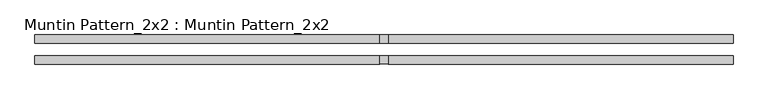
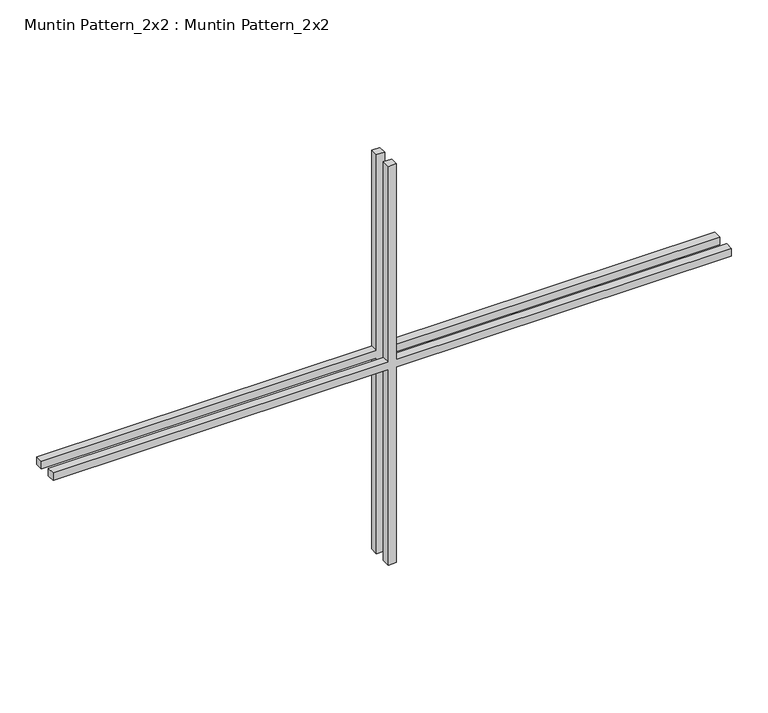
"""IFC4 building model written with IfcOpenShell, lengths in millimetres: proxy geometry, Muntin Pattern_2x2 : Muntin Pattern_2x2."""

from ifc_helpers import new_model, si_unit, frame, origin, place, context, project, spatial, polyline, outline, extrude, source, transform, mapped, element, save


def muntin_pattern_2x2_muntin_pattern_2x2_afeb4eca(model_context):
    return source(origin(), model_context, "Body", "SweptSolid", [
        extrude(outline(polyline([(338.1375, -6.35), (338.1375, -533.4), (325.4375, -533.4), (325.4375, -6.35), (0.0, -6.35), (0.0, 6.35), (325.4375, 6.35), (325.4375, 533.4), (338.1375, 533.4), (338.1375, 6.35), (663.575, 6.35), (663.575, -6.35), (338.1375, -6.35)])), frame((0.0, 9.525, 0.0), z_axis=(0.0, 1.0, 0.0), x_axis=(0.0, 0.0, 1.0)), (0.0, 0.0, 1.0), 12.7),
        extrude(outline(polyline([(338.1375, -6.35), (338.1375, -533.4), (325.4375, -533.4), (325.4375, -6.35), (0.0, -6.35), (0.0, 6.35), (325.4375, 6.35), (325.4375, 533.4), (338.1375, 533.4), (338.1375, 6.35), (663.575, 6.35), (663.575, -6.35), (338.1375, -6.35)])), frame((0.0, -22.225, 0.0), z_axis=(0.0, 1.0, 0.0), x_axis=(0.0, 0.0, 1.0)), (0.0, 0.0, 1.0), 12.7),
    ])


if __name__ == "__main__":
    model = new_model("IFC4")
    model_context = context("Model", 3, world=origin())
    ifc_project = project(units=[si_unit("LENGTHUNIT", "METRE", prefix="MILLI")], contexts=[model_context])
    site = spatial("IfcSite", under=ifc_project)
    building = spatial("IfcBuilding", under=site)
    placement = place(None, origin())
    muntin_pattern_2x2_muntin_pattern_2x2_shape = muntin_pattern_2x2_muntin_pattern_2x2_afeb4eca(model_context)
    element("IfcBuildingElementProxy", 1, Name="Muntin Pattern_2x2 : Muntin Pattern_2x2", ObjectType="Muntin Pattern_2x2 : Muntin Pattern_2x2", at=placement, inside=building, context=model_context, shape_type="MappedRepresentation", body=[
        mapped(muntin_pattern_2x2_muntin_pattern_2x2_shape, transform((0.0, 0.0, 0.0), x_axis=(1.0, 0.0, 0.0), y_axis=(0.0, 1.0, 0.0), z_axis=(0.0, 0.0, 1.0))),
    ])
    save(model, "model.ifc")

# Revit data of these elements
# Type "Muntin Pattern_2x2 : Muntin Pattern_2x2"
#   Width [instance default] = 4' - 0"
#   Thickness = 0' - 0 1/2"
#   Height [instance default] = 4' - 0"
#   Distance = 0' - 0 3/4"
#   Interior Material [instance default] = none
#   Exterior Material [instance default] = none
#   Default Elevation = 0
# Element 1 (IfcBuildingElementProxy, "Muntin Pattern_2x2 : Muntin Pattern_2x2")
#   Width = 3' - 6"
#   Height = 2' - 2 1/8"
#   Interior Material = Wood - Stained
#   Exterior Material = Clad - White
#   Materials on its faces: "Clad - White", "Wood - Stained"
# Materials
#   "Clad - White": class "Wood", colour RGB 242 242 238, transparency 0, Cost = 0
#   "Wood - Stained": class "Wood", colour RGB 224 178 126, transparency 0, Cost = 0
